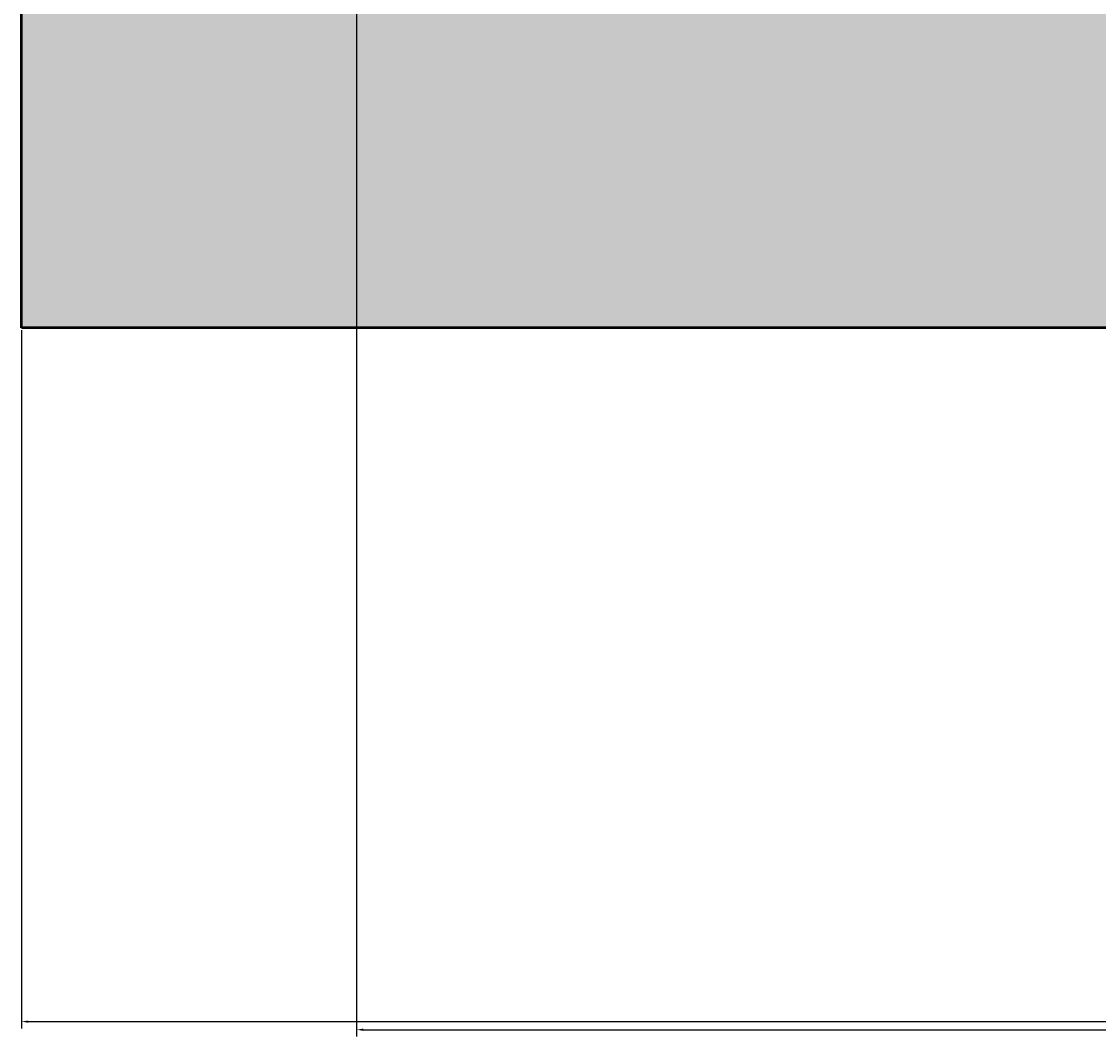
# Model space of a CAD drawing. Units: inches. Extents: x 2231 to 2461, y 2045 to 2455.
# Tile 1 of 95: x 2250 to 2279, y 2045 to 2072. Entities that reach past the tile are written whole.
import ezdxf

# ---------------------------------------------------------------- set-up
doc = ezdxf.new("R2010")
doc.units = ezdxf.units.IN
doc.layers.add('A-ANNO-DIMS', color=2, linetype='Continuous', lineweight=18)
doc.layers.add('A-WALL', color=7, linetype='Continuous', lineweight=50)
doc.layers.add('A-WALL-PATT', color=18, linetype='Continuous', lineweight=13, true_color=0x000000)
doc.styles.get("Standard").update_dxf_attribs({"font": 'arial.ttf'})
doc.dimstyles.get("Standard").update_dxf_attribs({"dimtxt": 0.18, "dimasz": 0.18, "dimexe": 0.18, "dimexo": 0.0625, "dimgap": 0.09, "dimtad": 0, "dimtih": 1, "dimtoh": 1, "dimdec": 4, "dimzin": 0, "dimdsep": 46, "dimtxsty": 'Standard', "dimcen": 0.09, "dimadec": 0, "dimazin": 0, "dimtfac": 1, "dimtdec": 4, "dimtofl": 0, "dimtmove": 0, "dimatfit": 3, "dimfxl": 1, "dimtolj": 1, "dimtzin": 0, "dimarcsym": 0})

# ---------------------------------------------------------------- blocks, each defined once
blk = doc.blocks.new('*D33')
at = {"layer": 'A-ANNO-DIMS', "color": 0, "lineweight": -2, "transparency": 16777216}
for p, q in [((2249.794, 2063.77), (2249.794, 2045.02)), ((2441.794, 2063.77), (2441.794, 2045.02)), ((2249.974, 2045.2), (2345.514, 2045.2)), ((2441.614, 2045.2), (2346.073, 2045.2))]:
    blk.add_line(p, q, dxfattribs=at)
at = {"layer": 'A-ANNO-DIMS', "color": 0, "transparency": 16777216}
for points in [[(2249.974, 2045.23), (2249.974, 2045.17), (2249.794, 2045.2)], [(2441.614, 2045.23), (2441.614, 2045.17), (2441.794, 2045.2)]]:
    blk.add_solid(points, dxfattribs=at)
at = {"layer": 'Defpoints', "color": 0, "transparency": 16777216}
for p in [(2249.794, 2063.833), (2441.794, 2063.833), (2249.794, 2045.2)]:
    blk.add_point(p, dxfattribs=at)
at = {"layer": 'A-ANNO-DIMS', "color": 0, "transparency": 16777216, "insert": (2345.794, 2045.2), "char_height": 0.18, "attachment_point": 5}
blk.add_mtext('\\A1;192', dxfattribs=at)
blk = doc.blocks.new('*D51')
at = {"layer": 'A-ANNO-DIMS', "color": 0, "lineweight": -2, "transparency": 16777216}
for p, q in [((2258.794, 2306.77), (2258.794, 2044.803)), ((2330.794, 2306.77), (2330.794, 2044.803)), ((2258.974, 2044.983), (2294.576, 2044.983)), ((2330.614, 2044.983), (2295.011, 2044.983))]:
    blk.add_line(p, q, dxfattribs=at)
at = {"layer": 'A-ANNO-DIMS', "color": 0, "transparency": 16777216}
for points in [[(2258.974, 2045.013), (2258.974, 2044.953), (2258.794, 2044.983)], [(2330.614, 2045.013), (2330.614, 2044.953), (2330.794, 2044.983)]]:
    blk.add_solid(points, dxfattribs=at)
at = {"layer": 'Defpoints', "color": 0, "transparency": 16777216}
for p in [(2258.794, 2306.833), (2330.794, 2306.833), (2330.794, 2044.983)]:
    blk.add_point(p, dxfattribs=at)
at = {"layer": 'A-ANNO-DIMS', "color": 0, "transparency": 16777216, "insert": (2294.794, 2044.983), "char_height": 0.18, "attachment_point": 5}
blk.add_mtext('\\A1;72', dxfattribs=at)

msp = doc.modelspace()

# ---------------------------------------------------------------- hatches: boundary and pattern name
at = {"layer": 'A-WALL-PATT'}
h = msp.add_hatch(color=256, dxfattribs=at)
h.dxf.hatch_style = 1
h.paths.add_polyline_path([(2441.7935, 2269.1535), (2432.7935, 2269.1535), (2432.7935, 2186.8328), (2396.7935, 2186.8328), (2396.7935, 2286.8328), (2394.7935, 2286.8328), (2394.7935, 2186.8328), (2334.7935, 2186.8328), (2334.7935, 2182.8328), (2432.7935, 2182.8328), (2432.7935, 2072.8328), (2416.6639, 2072.8328), (2416.6639, 2063.8328), (2441.7935, 2063.8328)])
h.paths.add_polyline_path([(2368.6639, 2072.8328), (2367.04, 2072.8328), (2330.7942, 2072.8328), (2330.7397, 2063.8328), (2368.6639, 2063.8328)])
h.paths.add_polyline_path([(2300.7392, 2068.3328), (2300.7392, 2072.8328), (2298.7935, 2072.8328), (2294.7935, 2072.8328), (2258.7935, 2072.8328), (2258.7935, 2120.8328), (2294.7935, 2120.8328), (2298.7935, 2120.8328), (2298.7935, 2128.8328), (2294.7935, 2128.8328), (2294.7935, 2124.8328), (2258.7935, 2124.8328), (2258.7935, 2182.8328), (2294.7935, 2182.8328), (2294.7935, 2174.8328), (2298.7935, 2174.8328), (2298.7935, 2182.8328), (2304.7935, 2182.8328), (2304.7935, 2186.8328), (2258.7935, 2186.8328), (2258.7935, 2221.999), (2249.7935, 2221.999), (2249.7935, 2063.8328), (2300.7392, 2063.8328)])
h.paths.add_polyline_path([(2391.9338, 2435.8328), (2333.82, 2435.8328), (2333.82, 2426.8328), (2368.7935, 2426.8328), (2368.7935, 2374.9508), (2368.7935, 2370.8328), (2372.3935, 2370.8328), (2372.7935, 2370.8328), (2372.7935, 2426.8328), (2391.9338, 2426.8328)])
h.paths.add_polyline_path([(2441.7935, 2435.8328), (2415.9338, 2435.8328), (2415.9338, 2426.8328), (2432.7935, 2426.8328), (2432.7935, 2334.8328), (2372.7935, 2334.8328), (2372.7935, 2346.8328), (2368.7935, 2346.8328), (2368.7935, 2306.8328), (2360.7935, 2306.8328), (2360.7935, 2302.8328), (2368.7935, 2302.8328), (2372.7935, 2302.8328), (2372.7935, 2330.8328), (2432.7935, 2330.8328), (2432.7935, 2317.1535), (2441.7935, 2317.1535)])
h.paths.add_polyline_path([(2285.82, 2435.8328), (2249.7935, 2435.8328), (2249.7935, 2269.999), (2258.7935, 2269.999), (2258.7935, 2302.8328), (2318.8168, 2302.8328), (2330.7935, 2302.8328), (2330.7935, 2306.8328), (2258.7935, 2306.8328), (2258.7935, 2426.8328), (2285.82, 2426.8328)])

# ---------------------------------------------------------------- linework, layer by layer
at = {"layer": 'A-WALL'}
msp.add_lwpolyline([(2300.7392, 2063.8328), (2249.7935, 2063.8328), (2249.7935, 2435.8328), (2441.7935, 2435.8328), (2441.7935, 2063.8328), (2330.7397, 2063.8328)], dxfattribs=at)

# ---------------------------------------------------------------- dimensions: what is measured, and where the dimension line sits
at = {"layer": 'A-ANNO-DIMS'}
dim = msp.add_linear_dim(base=(2330.7935, 2044.9825), p1=(2258.7935, 2306.8328), p2=(2330.7935, 2306.8328), dimstyle='Standard', override={"dimdec": 0, "dimlfac": 1, "dimrnd": 0, "dimzin": 0, "dimdsep": 46, "dimlunit": 2}, dxfattribs=at)
dim.commit()
dim.dimension.update_dxf_attribs({"geometry": '*D51', "text_midpoint": (2294.7935, 2044.9825)})
dim = msp.add_linear_dim(base=(2249.7935, 2045.2003), p1=(2441.7935, 2063.8328), p2=(2249.7935, 2063.8328), angle=180, dimstyle='Standard', override={"dimdec": 0, "dimlfac": 1, "dimrnd": 0, "dimzin": 0, "dimdsep": 46, "dimlunit": 2}, dxfattribs=at)
dim.commit()
dim.dimension.update_dxf_attribs({"geometry": '*D33', "text_midpoint": (2345.7935, 2045.2003)})

doc.saveas('drawing.dxf')
